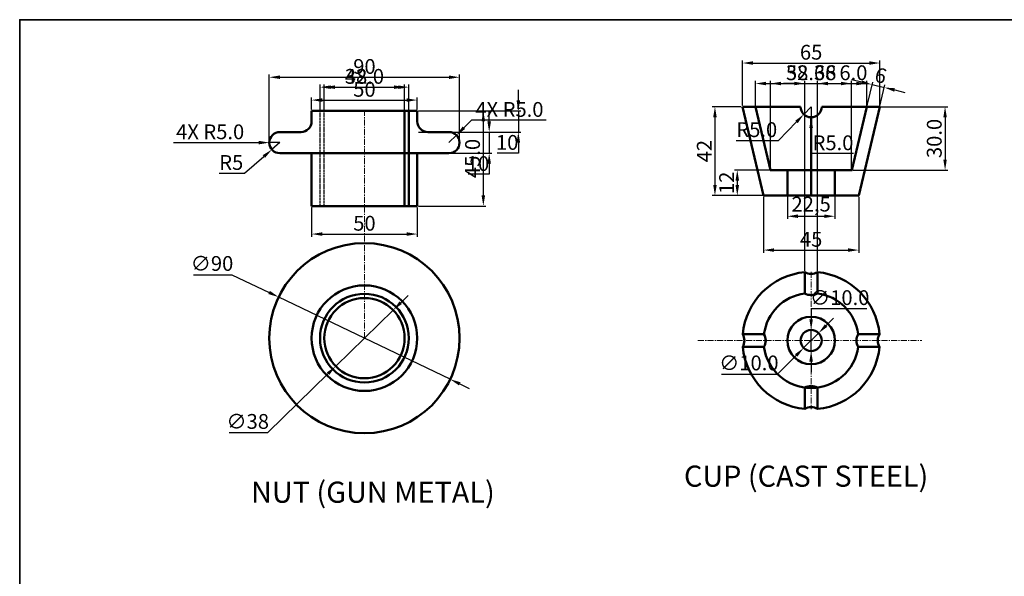
# Model space of a CAD drawing. Units: millimetres. Extents: x 4274 to 5106, y 2129 to 2785.
# Tile 2 of 4: x 4274 to 4740, y 2522 to 2785. Entities that reach past the tile are written whole.
import ezdxf

# ---------------------------------------------------------------- set-up
doc = ezdxf.new("R2010")
doc.units = ezdxf.units.MM
doc.header["$LTSCALE"] = 0.3
doc.linetypes.add('ACAD_ISO02W100', pattern=[15, 12, -3])
doc.linetypes.add('CENTER', pattern=[50.8, 31.75, -6.35, 6.35, -6.35])
for name, color, linetype, lineweight in [('M-CNTR', 1, 'CENTER', 18), ('M-DIMS', 2, 'Continuous', 25), ('M-HIDN', 8, 'ACAD_ISO02W100', 25), ('M-OUTL', 7, 'Continuous', 50), ('M-TEXT', 3, 'Continuous', 25), ('M-TTLB', 7, 'Continuous', 35)]:
    doc.layers.add(name, color=color, linetype=linetype, lineweight=lineweight)
doc.styles.get("Standard").update_dxf_attribs({"font": 'arial.ttf'})
doc.dimstyles.new('ISO-25', dxfattribs={"dimtxt": 7, "dimasz": 5, "dimexe": 1.25, "dimexo": 0.625, "dimtad": 1, "dimtoh": 1, "dimtxsty": 'Standard', "dimcen": 2.5, "dimadec": 0, "dimazin": 0, "dimtfac": 1, "dimtmove": 0, "dimatfit": 3, "dimfxl": 1, "dimarcsym": 0})

# ---------------------------------------------------------------- blocks, each defined once
blk = doc.blocks.new('*D10')
at = {"layer": 'Defpoints', "color": 0, "ltscale": 0.3, "transparency": 16777216}
for p in [(4482.08, 2757.92), (4392.08, 2726.98), (4482.08, 2726.98)]:
    blk.add_point(p, dxfattribs=at)
at = {"layer": 'M-DIMS', "color": 0, "lineweight": -2, "ltscale": 0.3, "transparency": 16777216}
for p, q in [((4392.08, 2727.6), (4392.08, 2759.17)), ((4482.08, 2727.6), (4482.08, 2759.17)), ((4397.08, 2757.92), (4477.08, 2757.92))]:
    blk.add_line(p, q, dxfattribs=at)
at = {"layer": 'M-DIMS', "color": 0, "ltscale": 0.3, "transparency": 16777216}
for points in [[(4397.08, 2758.76), (4397.08, 2757.09), (4392.08, 2757.92)], [(4477.08, 2758.76), (4477.08, 2757.09), (4482.08, 2757.92)]]:
    blk.add_solid(points, dxfattribs=at)
at = {"layer": 'M-DIMS', "color": 0, "ltscale": 0.3, "transparency": 16777216, "insert": (4437.08, 2762.12), "char_height": 7, "attachment_point": 5}
blk.add_mtext('90', dxfattribs=at)
blk = doc.blocks.new('*D11')
at = {"layer": 'Defpoints', "color": 0, "ltscale": 0.3, "transparency": 16777216}
for p in [(4462.08, 2747.11), (4412.08, 2741.98), (4462.08, 2741.98)]:
    blk.add_point(p, dxfattribs=at)
at = {"layer": 'M-DIMS', "color": 0, "lineweight": -2, "ltscale": 0.3, "transparency": 16777216}
for p, q in [((4412.08, 2742.6), (4412.08, 2748.36)), ((4417.08, 2747.11), (4457.08, 2747.11)), ((4462.08, 2742.6), (4462.08, 2748.36))]:
    blk.add_line(p, q, dxfattribs=at)
at = {"layer": 'M-DIMS', "color": 0, "ltscale": 0.3, "transparency": 16777216}
for points in [[(4417.08, 2747.95), (4417.08, 2746.28), (4412.08, 2747.11)], [(4457.08, 2747.95), (4457.08, 2746.28), (4462.08, 2747.11)]]:
    blk.add_solid(points, dxfattribs=at)
at = {"layer": 'M-DIMS', "color": 0, "ltscale": 0.3, "transparency": 16777216, "insert": (4437.08, 2751.31), "char_height": 7, "attachment_point": 5}
blk.add_mtext('50', dxfattribs=at)
blk = doc.blocks.new('*D12')
at = {"layer": 'Defpoints', "color": 0, "ltscale": 0.3, "transparency": 16777216}
for p in [(4412.08, 2696.98), (4462.08, 2696.98), (4462.08, 2683.71)]:
    blk.add_point(p, dxfattribs=at)
at = {"layer": 'M-DIMS', "color": 0, "lineweight": -2, "ltscale": 0.3, "transparency": 16777216}
for p, q in [((4412.08, 2696.35), (4412.08, 2682.46)), ((4462.08, 2696.35), (4462.08, 2682.46)), ((4417.08, 2683.71), (4457.08, 2683.71))]:
    blk.add_line(p, q, dxfattribs=at)
at = {"layer": 'M-DIMS', "color": 0, "ltscale": 0.3, "transparency": 16777216}
for points in [[(4417.08, 2684.54), (4417.08, 2682.88), (4412.08, 2683.71)], [(4457.08, 2684.54), (4457.08, 2682.88), (4462.08, 2683.71)]]:
    blk.add_solid(points, dxfattribs=at)
at = {"layer": 'M-DIMS', "color": 0, "ltscale": 0.3, "transparency": 16777216, "insert": (4437.08, 2687.91), "char_height": 7, "attachment_point": 5}
blk.add_mtext('50', dxfattribs=at)
blk = doc.blocks.new('*D13')
at = {"layer": 'Defpoints', "color": 0, "ltscale": 0.3, "transparency": 16777216}
for p in [(4397.08, 2726.98), (4393.3, 2723.7)]:
    blk.add_point(p, dxfattribs=at)
at = {"layer": 'M-DIMS', "color": 0, "lineweight": -2, "ltscale": 0.3, "transparency": 16777216}
for p, q in [((4397.08, 2726.98), (4393.3, 2723.7)), ((4380.36, 2712.5), (4389.52, 2720.43)), ((4368.39, 2712.5), (4380.36, 2712.5))]:
    blk.add_line(p, q, dxfattribs=at)
at = {"layer": 'M-DIMS', "color": 0, "ltscale": 0.3, "transparency": 16777216}
blk.add_solid([(4388.97, 2721.06), (4390.06, 2719.8), (4393.3, 2723.7)], dxfattribs=at)
at = {"layer": 'M-DIMS', "color": 0, "ltscale": 0.3, "transparency": 16777216, "insert": (4374.06, 2716.68), "char_height": 7, "attachment_point": 5}
blk.add_mtext('R5', dxfattribs=at)
blk = doc.blocks.new('*D14')
at = {"layer": 'Defpoints', "color": 0, "ltscale": 0.3, "transparency": 16777216}
for p in [(4477.08, 2731.98), (4477.08, 2721.98), (4496.11, 2721.98)]:
    blk.add_point(p, dxfattribs=at)
at = {"layer": 'M-DIMS', "color": 0, "lineweight": -2, "ltscale": 0.3, "transparency": 16777216}
for p, q in [((4496.11, 2736.98), (4496.11, 2741.98)), ((4477.7, 2731.98), (4497.36, 2731.98)), ((4496.11, 2731.98), (4496.11, 2721.98)), ((4477.7, 2721.98), (4497.36, 2721.98)), ((4496.11, 2716.98), (4496.11, 2711.98)), ((4496.11, 2711.98), (4486.14, 2711.98))]:
    blk.add_line(p, q, dxfattribs=at)
at = {"layer": 'M-DIMS', "color": 0, "ltscale": 0.3, "transparency": 16777216}
for points in [[(4495.28, 2736.98), (4496.94, 2736.98), (4496.11, 2731.98)], [(4495.28, 2716.98), (4496.94, 2716.98), (4496.11, 2721.98)]]:
    blk.add_solid(points, dxfattribs=at)
at = {"layer": 'M-DIMS', "color": 0, "ltscale": 0.3, "transparency": 16777216, "insert": (4490.81, 2716.17), "char_height": 7, "attachment_point": 5}
blk.add_mtext('10', dxfattribs=at)
blk = doc.blocks.new('*D15')
at = {"layer": 'Defpoints', "color": 0, "ltscale": 0.3, "transparency": 16777216}
for p in [(4462.08, 2741.98), (4462.08, 2731.98), (4509.9, 2731.98)]:
    blk.add_point(p, dxfattribs=at)
at = {"layer": 'M-DIMS', "color": 0, "lineweight": -2, "ltscale": 0.3, "transparency": 16777216}
for p, q in [((4509.9, 2746.98), (4509.9, 2751.98)), ((4462.7, 2741.98), (4511.15, 2741.98)), ((4509.9, 2741.98), (4509.9, 2731.98)), ((4462.7, 2731.98), (4511.15, 2731.98)), ((4509.9, 2726.98), (4509.9, 2721.98)), ((4509.9, 2721.98), (4499.94, 2721.98))]:
    blk.add_line(p, q, dxfattribs=at)
at = {"layer": 'M-DIMS', "color": 0, "ltscale": 0.3, "transparency": 16777216}
for points in [[(4509.07, 2746.98), (4510.74, 2746.98), (4509.9, 2741.98)], [(4509.07, 2726.98), (4510.74, 2726.98), (4509.9, 2731.98)]]:
    blk.add_solid(points, dxfattribs=at)
at = {"layer": 'M-DIMS', "color": 0, "ltscale": 0.3, "transparency": 16777216, "insert": (4504.61, 2726.17), "char_height": 7, "attachment_point": 5}
blk.add_mtext('10', dxfattribs=at)
blk = doc.blocks.new('*D16')
at = {"layer": 'Defpoints', "color": 0, "ltscale": 0.3, "transparency": 16777216}
for p in [(4396.5, 2653.89), (4477.66, 2614.98)]:
    blk.add_point(p, dxfattribs=at)
at = {"layer": 'M-DIMS', "color": 0, "lineweight": -2, "ltscale": 0.3, "transparency": 16777216}
for p, q in [((4356.15, 2664.48), (4374.39, 2664.48)), ((4374.39, 2664.48), (4391.99, 2656.05)), ((4477.66, 2614.98), (4396.5, 2653.89)), ((4482.17, 2612.82), (4486.67, 2610.66))]:
    blk.add_line(p, q, dxfattribs=at)
at = {"layer": 'M-DIMS', "color": 0, "ltscale": 0.3, "transparency": 16777216}
for points in [[(4392.35, 2656.8), (4391.63, 2655.3), (4396.5, 2653.89)], [(4482.53, 2613.57), (4481.81, 2612.07), (4477.66, 2614.98)]]:
    blk.add_solid(points, dxfattribs=at)
at = {"layer": 'M-DIMS', "color": 0, "ltscale": 0.3, "transparency": 16777216, "insert": (4364.96, 2668.88), "char_height": 7, "attachment_point": 5}
blk.add_mtext('∅90', dxfattribs=at)
blk = doc.blocks.new('*D17')
at = {"layer": 'Defpoints', "color": 0, "ltscale": 0.3, "transparency": 16777216}
for p in [(4450.67, 2647.71), (4423.49, 2621.16)]:
    blk.add_point(p, dxfattribs=at)
at = {"layer": 'M-DIMS', "color": 0, "lineweight": -2, "ltscale": 0.3, "transparency": 16777216}
for p, q in [((4454.25, 2651.2), (4457.82, 2654.7)), ((4450.67, 2647.71), (4423.49, 2621.16)), ((4391.3, 2589.73), (4419.91, 2617.67)), ((4373.02, 2589.73), (4391.3, 2589.73))]:
    blk.add_line(p, q, dxfattribs=at)
at = {"layer": 'M-DIMS', "color": 0, "ltscale": 0.3, "transparency": 16777216}
for points in [[(4453.67, 2651.8), (4454.83, 2650.61), (4450.67, 2647.71)], [(4419.33, 2618.26), (4420.49, 2617.07), (4423.49, 2621.16)]]:
    blk.add_solid(points, dxfattribs=at)
at = {"layer": 'M-DIMS', "color": 0, "ltscale": 0.3, "transparency": 16777216, "insert": (4381.85, 2594.12), "char_height": 7, "attachment_point": 5}
blk.add_mtext('∅38', dxfattribs=at)
blk = doc.blocks.new('*D18')
at = {"layer": 'Defpoints', "color": 0, "ltscale": 0.3, "transparency": 16777216}
for p in [(4680.93, 2764.66), (4615.93, 2743.95), (4680.93, 2743.95)]:
    blk.add_point(p, dxfattribs=at)
at = {"layer": 'M-DIMS', "color": 0, "lineweight": -2, "ltscale": 0.3, "transparency": 16777216}
for p, q in [((4615.93, 2744.58), (4615.93, 2765.91)), ((4620.93, 2764.66), (4675.93, 2764.66)), ((4680.93, 2744.58), (4680.93, 2765.91))]:
    blk.add_line(p, q, dxfattribs=at)
at = {"layer": 'M-DIMS', "color": 0, "ltscale": 0.3, "transparency": 16777216}
for points in [[(4620.93, 2765.49), (4620.93, 2763.82), (4615.93, 2764.66)], [(4675.93, 2765.49), (4675.93, 2763.82), (4680.93, 2764.66)]]:
    blk.add_solid(points, dxfattribs=at)
at = {"layer": 'M-DIMS', "color": 0, "ltscale": 0.3, "transparency": 16777216, "insert": (4648.43, 2768.86), "char_height": 7, "attachment_point": 5}
blk.add_mtext('65', dxfattribs=at)
blk = doc.blocks.new('*D19')
at = {"layer": 'Defpoints', "color": 0, "ltscale": 0.3, "transparency": 16777216}
for p in [(4683.09, 2753.06), (4671.19, 2728.95), (4677.02, 2727.56)]:
    blk.add_point(p, dxfattribs=at)
at = {"layer": 'M-DIMS', "color": 0, "lineweight": -2, "ltscale": 0.3, "transparency": 16777216}
for p, q in [((4672.39, 2755.6), (4667.53, 2756.76)), ((4671.33, 2729.56), (4677.55, 2755.66)), ((4677.17, 2728.17), (4683.38, 2754.27)), ((4677.26, 2754.45), (4683.09, 2753.06)), ((4687.96, 2751.9), (4692.82, 2750.74))]:
    blk.add_line(p, q, dxfattribs=at)
at = {"layer": 'M-DIMS', "color": 0, "ltscale": 0.3, "transparency": 16777216}
for points in [[(4672.59, 2756.41), (4672.2, 2754.79), (4677.26, 2754.45)], [(4688.15, 2752.71), (4687.76, 2751.09), (4683.09, 2753.06)]]:
    blk.add_solid(points, dxfattribs=at)
at = {"layer": 'M-DIMS', "color": 0, "ltscale": 0.3, "transparency": 16777216, "insert": (4681.15, 2757.84), "char_height": 7, "attachment_point": 5, "rotation": 346.6075}
blk.add_mtext('6', dxfattribs=at)
blk = doc.blocks.new('*D20')
at = {"layer": 'Defpoints', "color": 0, "ltscale": 0.3, "transparency": 16777216}
for p in [(4615.93, 2743.95), (4602.92, 2701.95), (4625.93, 2701.95)]:
    blk.add_point(p, dxfattribs=at)
at = {"layer": 'M-DIMS', "color": 0, "lineweight": -2, "ltscale": 0.3, "transparency": 16777216}
for p, q in [((4615.3, 2743.95), (4601.67, 2743.95)), ((4602.92, 2738.95), (4602.92, 2706.95)), ((4625.3, 2701.95), (4601.67, 2701.95))]:
    blk.add_line(p, q, dxfattribs=at)
at = {"layer": 'M-DIMS', "color": 0, "ltscale": 0.3, "transparency": 16777216}
for points in [[(4602.09, 2738.95), (4603.76, 2738.95), (4602.92, 2743.95)], [(4602.09, 2706.95), (4603.76, 2706.95), (4602.92, 2701.95)]]:
    blk.add_solid(points, dxfattribs=at)
at = {"layer": 'M-DIMS', "color": 0, "ltscale": 0.3, "transparency": 16777216, "insert": (4598.78, 2722.95), "char_height": 7, "attachment_point": 5, "rotation": 90}
blk.add_mtext('42', dxfattribs=at)
blk = doc.blocks.new('*D21')
at = {"layer": 'Defpoints', "color": 0, "ltscale": 0.3, "transparency": 16777216}
for p in [(4637.18, 2713.95), (4613.49, 2701.95), (4637.18, 2701.95)]:
    blk.add_point(p, dxfattribs=at)
at = {"layer": 'M-DIMS', "color": 0, "lineweight": -2, "ltscale": 0.3, "transparency": 16777216}
for p, q in [((4636.55, 2713.95), (4612.24, 2713.95)), ((4613.49, 2708.95), (4613.49, 2706.95)), ((4636.55, 2701.95), (4612.24, 2701.95))]:
    blk.add_line(p, q, dxfattribs=at)
at = {"layer": 'M-DIMS', "color": 0, "ltscale": 0.3, "transparency": 16777216}
for points in [[(4612.65, 2708.95), (4614.32, 2708.95), (4613.49, 2713.95)], [(4612.65, 2706.95), (4614.32, 2706.95), (4613.49, 2701.95)]]:
    blk.add_solid(points, dxfattribs=at)
at = {"layer": 'M-DIMS', "color": 0, "ltscale": 0.3, "transparency": 16777216, "insert": (4609.35, 2707.95), "char_height": 7, "attachment_point": 5, "rotation": 90}
blk.add_mtext('12', dxfattribs=at)
blk = doc.blocks.new('*D22')
at = {"layer": 'Defpoints', "color": 0, "ltscale": 0.3, "transparency": 16777216}
for p in [(4625.93, 2701.95), (4670.93, 2701.95), (4670.93, 2676.12)]:
    blk.add_point(p, dxfattribs=at)
at = {"layer": 'M-DIMS', "color": 0, "lineweight": -2, "ltscale": 0.3, "transparency": 16777216}
for p, q in [((4625.93, 2701.33), (4625.93, 2674.87)), ((4670.93, 2701.33), (4670.93, 2674.87)), ((4630.93, 2676.12), (4665.93, 2676.12))]:
    blk.add_line(p, q, dxfattribs=at)
at = {"layer": 'M-DIMS', "color": 0, "ltscale": 0.3, "transparency": 16777216}
for points in [[(4630.93, 2676.96), (4630.93, 2675.29), (4625.93, 2676.12)], [(4665.93, 2676.96), (4665.93, 2675.29), (4670.93, 2676.12)]]:
    blk.add_solid(points, dxfattribs=at)
at = {"layer": 'M-DIMS', "color": 0, "ltscale": 0.3, "transparency": 16777216, "insert": (4648.43, 2680.31), "char_height": 7, "attachment_point": 5}
blk.add_mtext('45', dxfattribs=at)
blk = doc.blocks.new('*D23')
at = {"layer": 'Defpoints', "color": 0, "ltscale": 0.3, "transparency": 16777216}
for p in [(4637.18, 2701.95), (4659.68, 2701.95), (4659.68, 2692.13)]:
    blk.add_point(p, dxfattribs=at)
at = {"layer": 'M-DIMS', "color": 0, "lineweight": -2, "ltscale": 0.3, "transparency": 16777216}
for p, q in [((4637.18, 2701.33), (4637.18, 2690.88)), ((4659.68, 2701.33), (4659.68, 2690.88)), ((4642.18, 2692.13), (4654.68, 2692.13))]:
    blk.add_line(p, q, dxfattribs=at)
at = {"layer": 'M-DIMS', "color": 0, "ltscale": 0.3, "transparency": 16777216}
for points in [[(4642.18, 2692.97), (4642.18, 2691.3), (4637.18, 2692.13)], [(4654.68, 2692.97), (4654.68, 2691.3), (4659.68, 2692.13)]]:
    blk.add_solid(points, dxfattribs=at)
at = {"layer": 'M-DIMS', "color": 0, "ltscale": 0.3, "transparency": 16777216, "insert": (4648.43, 2696.96), "char_height": 7, "attachment_point": 5}
blk.add_mtext('22,5', dxfattribs=at)
blk = doc.blocks.new('*D53')
at = {"layer": 'Defpoints', "color": 0, "ltscale": 0.3, "transparency": 16777216}
for p in [(4462.08, 2741.98), (4462.08, 2696.98), (4493.33, 2696.98)]:
    blk.add_point(p, dxfattribs=at)
at = {"layer": 'M-DIMS', "color": 0, "lineweight": -2, "ltscale": 0.3, "transparency": 16777216}
for p, q in [((4462.7, 2741.98), (4494.58, 2741.98)), ((4493.33, 2736.98), (4493.33, 2701.98)), ((4462.7, 2696.98), (4494.58, 2696.98))]:
    blk.add_line(p, q, dxfattribs=at)
at = {"layer": 'M-DIMS', "color": 0, "ltscale": 0.3, "transparency": 16777216}
for points in [[(4492.49, 2736.98), (4494.16, 2736.98), (4493.33, 2741.98)], [(4492.49, 2701.98), (4494.16, 2701.98), (4493.33, 2696.98)]]:
    blk.add_solid(points, dxfattribs=at)
at = {"layer": 'M-DIMS', "color": 0, "ltscale": 0.3, "transparency": 16777216, "insert": (4489.13, 2719.48), "char_height": 7, "attachment_point": 5, "rotation": 90}
blk.add_mtext('45.0', dxfattribs=at)
blk = doc.blocks.new('*D54')
at = {"layer": 'Defpoints', "color": 0, "ltscale": 0.3, "transparency": 16777216}
for p in [(4456.08, 2753.23), (4418.08, 2741.98), (4456.08, 2741.98)]:
    blk.add_point(p, dxfattribs=at)
at = {"layer": 'M-DIMS', "color": 0, "lineweight": -2, "ltscale": 0.3, "transparency": 16777216}
for p, q in [((4418.08, 2742.6), (4418.08, 2754.48)), ((4456.08, 2742.6), (4456.08, 2754.48)), ((4423.08, 2753.23), (4451.08, 2753.23))]:
    blk.add_line(p, q, dxfattribs=at)
at = {"layer": 'M-DIMS', "color": 0, "ltscale": 0.3, "transparency": 16777216}
for points in [[(4423.08, 2754.06), (4423.08, 2752.39), (4418.08, 2753.23)], [(4451.08, 2754.06), (4451.08, 2752.39), (4456.08, 2753.23)]]:
    blk.add_solid(points, dxfattribs=at)
at = {"layer": 'M-DIMS', "color": 0, "ltscale": 0.3, "transparency": 16777216, "insert": (4437.08, 2757.43), "char_height": 7, "attachment_point": 5}
blk.add_mtext('38.0', dxfattribs=at)
blk = doc.blocks.new('*D55')
at = {"layer": 'Defpoints', "color": 0, "ltscale": 0.3, "transparency": 16777216}
for p in [(4458.08, 2753.23), (4416.08, 2741.98), (4458.08, 2741.98)]:
    blk.add_point(p, dxfattribs=at)
at = {"layer": 'M-DIMS', "color": 0, "lineweight": -2, "ltscale": 0.3, "transparency": 16777216}
for p, q in [((4416.08, 2742.6), (4416.08, 2754.48)), ((4458.08, 2742.6), (4458.08, 2754.48)), ((4421.08, 2753.23), (4453.08, 2753.23))]:
    blk.add_line(p, q, dxfattribs=at)
at = {"layer": 'M-DIMS', "color": 0, "ltscale": 0.3, "transparency": 16777216}
for points in [[(4421.08, 2754.06), (4421.08, 2752.39), (4416.08, 2753.23)], [(4453.08, 2754.06), (4453.08, 2752.39), (4458.08, 2753.23)]]:
    blk.add_solid(points, dxfattribs=at)
at = {"layer": 'M-DIMS', "color": 0, "ltscale": 0.3, "transparency": 16777216, "insert": (4437.08, 2757.42), "char_height": 7, "attachment_point": 5}
blk.add_mtext('42.0', dxfattribs=at)
blk = doc.blocks.new('*D56')
at = {"layer": 'Defpoints', "color": 0, "ltscale": 0.3, "transparency": 16777216}
for p in [(4667.61, 2754.95), (4629.24, 2713.95), (4667.61, 2713.95)]:
    blk.add_point(p, dxfattribs=at)
at = {"layer": 'M-DIMS', "color": 0, "lineweight": -2, "ltscale": 0.3, "transparency": 16777216}
for p, q in [((4629.24, 2714.58), (4629.24, 2756.2)), ((4634.24, 2754.95), (4662.61, 2754.95)), ((4667.61, 2714.58), (4667.61, 2756.2))]:
    blk.add_line(p, q, dxfattribs=at)
at = {"layer": 'M-DIMS', "color": 0, "ltscale": 0.3, "transparency": 16777216}
for points in [[(4634.24, 2755.78), (4634.24, 2754.12), (4629.24, 2754.95)], [(4662.61, 2755.78), (4662.61, 2754.12), (4667.61, 2754.95)]]:
    blk.add_solid(points, dxfattribs=at)
at = {"layer": 'M-DIMS', "color": 0, "ltscale": 0.3, "transparency": 16777216, "insert": (4648.43, 2759.15), "char_height": 7, "attachment_point": 5}
blk.add_mtext('38.38', dxfattribs=at)
blk = doc.blocks.new('*D57')
at = {"layer": 'Defpoints', "color": 0, "ltscale": 0.3, "transparency": 16777216}
for p in [(4674.76, 2754.95), (4622.09, 2743.95), (4674.76, 2743.95)]:
    blk.add_point(p, dxfattribs=at)
at = {"layer": 'M-DIMS', "color": 0, "lineweight": -2, "ltscale": 0.3, "transparency": 16777216}
for p, q in [((4622.09, 2744.58), (4622.09, 2756.2)), ((4627.09, 2754.95), (4669.76, 2754.95)), ((4674.76, 2744.58), (4674.76, 2756.2))]:
    blk.add_line(p, q, dxfattribs=at)
at = {"layer": 'M-DIMS', "color": 0, "ltscale": 0.3, "transparency": 16777216}
for points in [[(4627.09, 2755.78), (4627.09, 2754.12), (4622.09, 2754.95)], [(4669.76, 2755.78), (4669.76, 2754.12), (4674.76, 2754.95)]]:
    blk.add_solid(points, dxfattribs=at)
at = {"layer": 'M-DIMS', "color": 0, "ltscale": 0.3, "transparency": 16777216, "insert": (4648.43, 2759.15), "char_height": 7, "attachment_point": 5}
blk.add_mtext('52.66', dxfattribs=at)
blk = doc.blocks.new('*D58')
at = {"layer": 'Defpoints', "color": 0, "ltscale": 0.3, "transparency": 16777216}
for p in [(4674.76, 2743.95), (4667.61, 2713.95), (4711.8, 2713.95)]:
    blk.add_point(p, dxfattribs=at)
at = {"layer": 'M-DIMS', "color": 0, "lineweight": -2, "ltscale": 0.3, "transparency": 16777216}
for p, q in [((4675.38, 2743.95), (4713.05, 2743.95)), ((4711.8, 2738.95), (4711.8, 2718.95)), ((4668.24, 2713.95), (4713.05, 2713.95))]:
    blk.add_line(p, q, dxfattribs=at)
at = {"layer": 'M-DIMS', "color": 0, "ltscale": 0.3, "transparency": 16777216}
for points in [[(4710.97, 2738.95), (4712.63, 2738.95), (4711.8, 2743.95)], [(4710.97, 2718.95), (4712.63, 2718.95), (4711.8, 2713.95)]]:
    blk.add_solid(points, dxfattribs=at)
at = {"layer": 'M-DIMS', "color": 0, "ltscale": 0.3, "transparency": 16777216, "insert": (4707.6, 2728.95), "char_height": 7, "attachment_point": 5, "rotation": 90}
blk.add_mtext('30.0', dxfattribs=at)
blk = doc.blocks.new('*D59')
at = {"layer": 'Defpoints', "color": 0, "ltscale": 0.3, "transparency": 16777216}
for p in [(4651.43, 2754.95), (4645.43, 2665.68), (4651.43, 2665.68)]:
    blk.add_point(p, dxfattribs=at)
at = {"layer": 'M-DIMS', "color": 0, "lineweight": -2, "ltscale": 0.3, "transparency": 16777216}
for p, q in [((4640.43, 2754.95), (4635.43, 2754.95)), ((4645.43, 2666.3), (4645.43, 2756.2)), ((4645.43, 2754.95), (4651.43, 2754.95)), ((4651.43, 2666.3), (4651.43, 2756.2)), ((4656.43, 2754.95), (4675.43, 2754.95))]:
    blk.add_line(p, q, dxfattribs=at)
at = {"layer": 'M-DIMS', "color": 0, "ltscale": 0.3, "transparency": 16777216}
for points in [[(4640.43, 2755.78), (4640.43, 2754.12), (4645.43, 2754.95)], [(4656.43, 2755.78), (4656.43, 2754.12), (4651.43, 2754.95)]]:
    blk.add_solid(points, dxfattribs=at)
at = {"layer": 'M-DIMS', "color": 0, "ltscale": 0.3, "transparency": 16777216, "insert": (4668.43, 2759.15), "char_height": 7, "attachment_point": 5}
blk.add_mtext('6.0', dxfattribs=at)
blk = doc.blocks.new('*D70')
at = {"layer": 'Defpoints', "color": 0, "ltscale": 0.3, "transparency": 16777216}
for p in [(4392.08, 2726.98), (4397.08, 2726.98)]:
    blk.add_point(p, dxfattribs=at)
at = {"layer": 'M-DIMS', "color": 0, "lineweight": -2, "ltscale": 0.3, "transparency": 16777216}
for p, q in [((4346.71, 2726.99), (4382.08, 2726.99)), ((4382.08, 2726.99), (4387.08, 2726.98)), ((4397.08, 2726.98), (4392.08, 2726.98))]:
    blk.add_line(p, q, dxfattribs=at)
at = {"layer": 'M-DIMS', "color": 0, "ltscale": 0.3, "transparency": 16777216}
blk.add_solid([(4387.08, 2727.82), (4387.08, 2726.15), (4392.08, 2726.98)], dxfattribs=at)
at = {"layer": 'M-DIMS', "color": 0, "ltscale": 0.3, "transparency": 16777216, "insert": (4364.08, 2731.19), "char_height": 7, "attachment_point": 5}
blk.add_mtext('4X R5.0', dxfattribs=at)
blk = doc.blocks.new('*D71')
at = {"layer": 'Defpoints', "color": 0, "ltscale": 0.3, "transparency": 16777216}
for p in [(4648.43, 2743.95), (4648.43, 2738.95)]:
    blk.add_point(p, dxfattribs=at)
at = {"layer": 'M-DIMS', "color": 0, "lineweight": -2, "ltscale": 0.3, "transparency": 16777216}
for p, q in [((4648.43, 2743.95), (4648.43, 2738.95)), ((4648.45, 2721.8), (4648.43, 2733.95)), ((4668.49, 2721.8), (4648.45, 2721.8))]:
    blk.add_line(p, q, dxfattribs=at)
at = {"layer": 'M-DIMS', "color": 0, "ltscale": 0.3, "transparency": 16777216}
blk.add_solid([(4649.27, 2733.95), (4647.6, 2733.95), (4648.43, 2738.95)], dxfattribs=at)
at = {"layer": 'M-DIMS', "color": 0, "ltscale": 0.3, "transparency": 16777216, "insert": (4658.78, 2726), "char_height": 7, "attachment_point": 5}
blk.add_mtext('R5.0', dxfattribs=at)
blk = doc.blocks.new('*D72')
at = {"layer": 'Defpoints', "color": 0, "ltscale": 0.3, "transparency": 16777216}
for p in [(4648.43, 2638.32), (4648.42, 2628.32)]:
    blk.add_point(p, dxfattribs=at)
at = {"layer": 'M-DIMS', "color": 0, "lineweight": -2, "ltscale": 0.3, "transparency": 16777216}
for p, q in [((4648.44, 2648.32), (4648.43, 2643.32)), ((4674.84, 2648.32), (4648.44, 2648.32)), ((4648.42, 2628.32), (4648.43, 2638.32)), ((4648.42, 2623.32), (4648.41, 2618.32))]:
    blk.add_line(p, q, dxfattribs=at)
at = {"layer": 'M-DIMS', "color": 0, "ltscale": 0.3, "transparency": 16777216}
for points in [[(4647.6, 2643.32), (4649.27, 2643.32), (4648.43, 2638.32)], [(4647.58, 2623.32), (4649.25, 2623.32), (4648.42, 2628.32)]]:
    blk.add_solid(points, dxfattribs=at)
at = {"layer": 'M-DIMS', "color": 0, "ltscale": 0.3, "transparency": 16777216, "insert": (4661.95, 2652.71), "char_height": 7, "attachment_point": 5}
blk.add_mtext('∅10.0', dxfattribs=at)
blk = doc.blocks.new('*D87')
at = {"layer": 'Defpoints', "color": 0, "ltscale": 0.3, "transparency": 16777216}
for p in [(4480.61, 2730.51), (4477.08, 2726.98)]:
    blk.add_point(p, dxfattribs=at)
at = {"layer": 'M-DIMS', "color": 0, "lineweight": -2, "ltscale": 0.3, "transparency": 16777216}
for p, q in [((4487.68, 2737.59), (4484.15, 2734.05)), ((4523.05, 2737.59), (4487.68, 2737.59)), ((4477.08, 2726.98), (4480.61, 2730.51))]:
    blk.add_line(p, q, dxfattribs=at)
at = {"layer": 'M-DIMS', "color": 0, "ltscale": 0.3, "transparency": 16777216}
blk.add_solid([(4483.56, 2734.64), (4484.74, 2733.46), (4480.61, 2730.51)], dxfattribs=at)
at = {"layer": 'M-DIMS', "color": 0, "ltscale": 0.3, "transparency": 16777216, "insert": (4505.68, 2741.78), "char_height": 7, "attachment_point": 5}
blk.add_mtext('4X R5.0', dxfattribs=at)
blk = doc.blocks.new('*D88')
at = {"layer": 'Defpoints', "color": 0, "ltscale": 0.3, "transparency": 16777216}
for p in [(4644.95, 2740.35), (4648.43, 2743.95)]:
    blk.add_point(p, dxfattribs=at)
at = {"layer": 'M-DIMS', "color": 0, "lineweight": -2, "ltscale": 0.3, "transparency": 16777216}
for p, q in [((4648.43, 2743.95), (4644.95, 2740.35)), ((4633.05, 2728.01), (4641.48, 2736.75)), ((4613, 2728.01), (4633.05, 2728.01))]:
    blk.add_line(p, q, dxfattribs=at)
at = {"layer": 'M-DIMS', "color": 0, "ltscale": 0.3, "transparency": 16777216}
blk.add_solid([(4640.88, 2737.33), (4642.08, 2736.18), (4644.95, 2740.35)], dxfattribs=at)
at = {"layer": 'M-DIMS', "color": 0, "ltscale": 0.3, "transparency": 16777216, "insert": (4622.71, 2732.21), "char_height": 7, "attachment_point": 5}
blk.add_mtext('R5.0', dxfattribs=at)
blk = doc.blocks.new('*D89')
at = {"layer": 'Defpoints', "color": 0, "ltscale": 0.3, "transparency": 16777216}
for p in [(4651.97, 2636.85), (4644.89, 2629.79)]:
    blk.add_point(p, dxfattribs=at)
at = {"layer": 'M-DIMS', "color": 0, "lineweight": -2, "ltscale": 0.3, "transparency": 16777216}
for p, q in [((4655.51, 2640.38), (4659.04, 2643.91)), ((4651.97, 2636.85), (4644.89, 2629.79)), ((4632.47, 2617.4), (4641.35, 2626.25)), ((4606.07, 2617.4), (4632.47, 2617.4))]:
    blk.add_line(p, q, dxfattribs=at)
at = {"layer": 'M-DIMS', "color": 0, "ltscale": 0.3, "transparency": 16777216}
for points in [[(4654.92, 2640.97), (4656.09, 2639.79), (4651.97, 2636.85)], [(4640.76, 2626.84), (4641.93, 2625.66), (4644.89, 2629.79)]]:
    blk.add_solid(points, dxfattribs=at)
at = {"layer": 'M-DIMS', "color": 0, "ltscale": 0.3, "transparency": 16777216, "insert": (4618.96, 2621.79), "char_height": 7, "attachment_point": 5}
blk.add_mtext('∅10.0', dxfattribs=at)

msp = doc.modelspace()

# ---------------------------------------------------------------- linework, layer by layer
at = {"layer": 'M-CNTR', "ltscale": 0.3}
for p, q in [((4437.0779, 2634.4352), (4437.0779, 2741.9752)), ((4648.4255, 2665.817), (4648.4255, 2600.817)), ((4594.8615, 2633.317), (4700.8, 2633.317))]:
    msp.add_line(p, q, dxfattribs=at)
at = {"layer": 'M-HIDN', "ltscale": 0.3}
for p, q in [((4416.0779, 2696.9752), (4416.0779, 2741.9752)), ((4418.0779, 2696.9752), (4418.0779, 2741.9752))]:
    msp.add_line(p, q, dxfattribs=at)
at = {"layer": 'M-OUTL', "ltscale": 0.3}
for p, q in [((4437.0779, 2741.9752), (4412.0779, 2741.9752)), ((4437.0779, 2741.9752), (4412.0779, 2741.9752)), ((4412.0779, 2741.9752), (4412.0779, 2736.9752)), ((4437.0779, 2741.9752), (4462.0779, 2741.9752)), ((4456.0779, 2696.9752), (4456.0779, 2741.9752)), ((4458.0779, 2696.9752), (4458.0779, 2741.9752)), ((4462.0779, 2736.9752), (4462.0779, 2741.9752)), ((4615.9255, 2743.9507), (4625.9255, 2701.9507)), ((4643.4255, 2743.9507), (4615.9255, 2743.9507)), ((4622.0932, 2743.9507), (4629.2361, 2713.9507)), ((4643.4255, 2743.9507), (4625.9255, 2743.9507)), ((4653.4255, 2743.9507), (4680.9255, 2743.9507)), ((4680.9255, 2743.9507), (4653.4255, 2743.9507)), ((4667.6149, 2713.9507), (4674.7578, 2743.9507)), ((4670.9255, 2701.9507), (4680.9255, 2743.9507)), ((4648.4255, 2738.9507), (4648.4255, 2701.9507)), ((4397.0779, 2731.9752), (4407.0779, 2731.9752)), ((4467.0779, 2731.9752), (4477.0779, 2731.9752)), ((4397.0779, 2721.9752), (4477.0779, 2721.9752)), ((4412.0779, 2721.9752), (4412.0779, 2696.9752)), ((4462.0779, 2696.9752), (4462.0779, 2721.9752)), ((4629.0684, 2713.9507), (4667.7826, 2713.9507)), ((4659.6755, 2713.9507), (4637.1755, 2713.9507)), ((4637.1755, 2713.9507), (4637.1755, 2701.9507)), ((4659.6755, 2713.9507), (4659.6755, 2701.9507)), ((4648.4255, 2701.9507), (4625.9255, 2701.9507)), ((4625.9255, 2701.9507), (4670.9255, 2701.9507)), ((4659.6755, 2701.9507), (4637.1755, 2701.9507)), ((4648.4255, 2701.9507), (4670.9255, 2701.9507)), ((4648.4255, 2701.9507), (4659.6755, 2701.9507)), ((4412.0779, 2696.9752), (4462.0779, 2696.9752)), ((4645.4255, 2665.6783), (4645.4255, 2655.6162)), ((4651.4255, 2665.6783), (4651.4255, 2655.6162)), ((4616.0643, 2636.317), (4626.1264, 2636.317)), ((4680.7867, 2636.317), (4670.7246, 2636.317)), ((4616.0643, 2630.317), (4626.1264, 2630.317)), ((4680.7867, 2630.317), (4670.7246, 2630.317)), ((4645.4255, 2600.9558), (4645.4255, 2611.0179)), ((4645.4255, 2611.0179), (4645.4255, 2600.9558)), ((4651.4255, 2600.9558), (4651.4255, 2611.0179)), ((4651.4255, 2611.0179), (4651.4255, 2600.9558))]:
    msp.add_line(p, q, dxfattribs=at)
for centre, radius in [((4437.0779, 2634.4352), 45), ((4437.0779, 2634.4352), 25), ((4437.0779, 2634.4352), 21), ((4437.0779, 2634.4352), 19), ((4648.4255, 2633.317), 11.25), ((4648.4255, 2633.317), 5)]:
    msp.add_circle(centre, radius, dxfattribs=at)
for centre, radius, start, end in [((4648.4255, 2743.9507), 5, 180, 0), ((4407.0779, 2736.9752), 5, 270, 0), ((4467.0779, 2736.9752), 5, 180, 270), ((4397.0779, 2726.9752), 5, 90, 270), ((4477.0779, 2726.9752), 5, 270, 90), ((4648.4255, 2633.317), 32.5, 95.296381, 174.703619), ((4648.4255, 2670.8744), 6, 240, 300), ((4648.4255, 2633.317), 32.5, 5.296381, 84.703619), ((4648.4255, 2633.317), 22.5, 97.662256, 172.337744), ((4648.4255, 2660.8123), 6, 240, 300), ((4648.4255, 2633.317), 22.5, 7.662256, 82.337744), ((4610.8681, 2633.317), 6, 330, 30), ((4620.9302, 2633.317), 6, 330, 30), ((4675.9208, 2633.317), 6, 150, 210), ((4685.9829, 2633.317), 6, 150, 210), ((4648.4255, 2633.317), 32.5, 185.296381, 264.703619), ((4648.4255, 2633.317), 22.5, 187.662256, 352.337744), ((4648.4255, 2633.317), 32.5, 275.296381, 354.703619), ((4648.4255, 2605.8218), 6, 60, 120), ((4648.4255, 2595.7597), 6, 60, 120)]:
    msp.add_arc(centre, radius, start, end, dxfattribs=at)
at = {"layer": 'M-TTLB', "ltscale": 0.3}
msp.add_lwpolyline([(5077.4601, 2139.9092), (4273.9655, 2139.9092), (4273.9655, 2785.1666), (5077.4601, 2785.1666)], close=True, dxfattribs=at)

# ---------------------------------------------------------------- texts
at = {"layer": 'M-TEXT', "ltscale": 0.3, "char_height": 10, "attachment_point": 1}
for s, width, insert in [('CUP (CAST STEEL)', 131.81659, (4588.2651, 2574.124)), ('NUT (GUN METAL)', 126.863962, (4383.4379, 2566.5278))]:
    msp.add_mtext_dynamic_manual_height_columns(s, width=width, gutter_width=12.5, heights=[0], dxfattribs=dict(at, insert=insert))

# ---------------------------------------------------------------- dimensions: what is measured, and where the dimension line sits
at = {"layer": 'M-DIMS', "ltscale": 0.3}
dim = msp.add_linear_dim(base=(4680.9255, 2764.6565), p1=(4615.9255, 2743.9507), p2=(4680.9255, 2743.9507), dimstyle='ISO-25', override={"dimclrd": 0, "dimclre": 0, "dimclrt": 0}, dxfattribs=at)
dim.commit()
dim.dimension.update_dxf_attribs({"geometry": '*D18', "text_midpoint": (4648.4255, 2764.6565), "dimtype": 160})
for base, p1, p2, override, picture, middle in [((4482.0779, 2757.9235), (4392.0779, 2726.9752), (4482.0779, 2726.9752), {"dimclrd": 0, "dimclre": 0, "dimclrt": 0}, '*D10', (4437.0779, 2762.1225)), ((4674.7578, 2754.9507), (4622.0932, 2743.9507), (4674.7578, 2743.9507), {"dimdec": 2, "dimlfac": 1, "dimrnd": 0, "dimzin": 0, "dimdsep": 46, "dimlunit": 2}, '*D57', (4648.4255, 2759.1498)), ((4667.6149, 2754.9507), (4629.2361, 2713.9507), (4667.6149, 2713.9507), {"dimdec": 2, "dimlfac": 1, "dimrnd": 0, "dimzin": 0, "dimdsep": 46, "dimlunit": 2}, '*D56', (4648.4255, 2759.1521)), ((4651.4255, 2754.9507), (4645.4255, 2665.6783), (4651.4255, 2665.6783), {"dimdec": 1, "dimlfac": 1, "dimrnd": 0, "dimzin": 0, "dimdsep": 46, "dimlunit": 2}, '*D59', (4668.4298, 2759.1498)), ((4458.0779, 2753.2252), (4416.0779, 2741.9752), (4458.0779, 2741.9752), {"dimdec": 1, "dimlfac": 1, "dimrnd": 0, "dimzin": 0, "dimdsep": 46, "dimlunit": 2}, '*D55', (4437.0779, 2757.4242)), ((4456.0779, 2753.2252), (4418.0779, 2741.9752), (4456.0779, 2741.9752), {"dimdec": 1, "dimlfac": 1, "dimrnd": 0, "dimzin": 0, "dimdsep": 46, "dimlunit": 2}, '*D54', (4437.0779, 2757.4266)), ((4462.0779, 2747.1133), (4412.0779, 2741.9752), (4462.0779, 2741.9752), {"dimclrd": 0, "dimclre": 0, "dimclrt": 0}, '*D11', (4437.0779, 2751.3123)), ((4670.9255, 2676.1229), (4625.9255, 2701.9507), (4670.9255, 2701.9507), {"dimclrd": 0, "dimclre": 0, "dimclrt": 0}, '*D22', (4648.4255, 2680.3076)), ((4659.6755, 2692.1324), (4637.1755, 2701.9507), (4659.6755, 2701.9507), {"dimclrd": 0, "dimclre": 0, "dimclrt": 0}, '*D23', (4648.4255, 2696.964)), ((4462.0779, 2683.7109), (4412.0779, 2696.9752), (4462.0779, 2696.9752), {"dimclrd": 0, "dimclre": 0, "dimclrt": 0}, '*D12', (4437.0779, 2687.9099))]:
    dim = msp.add_linear_dim(base=base, p1=p1, p2=p2, dimstyle='ISO-25', override=override, dxfattribs=at)
    dim.commit()
    dim.dimension.update_dxf_attribs({"geometry": picture, "text_midpoint": middle})
for p1, p2, distance, picture, middle in [((4671.1863, 2728.9507), (4677.0232, 2727.561), 26.2077, '*D19', (4681.1476, 2757.8358)), ((4462.0779, 2741.9752), (4462.0779, 2731.9752), 47.827, '*D15', (4504.6077, 2726.1742)), ((4477.0779, 2731.9752), (4477.0779, 2721.9752), 19.0335, '*D14', (4490.8142, 2716.1742))]:
    dim = msp.add_aligned_dim(p1=p1, p2=p2, distance=distance, dimstyle='ISO-25', override={"dimclrd": 0, "dimclre": 0, "dimclrt": 0}, dxfattribs=at)
    dim.commit()
    dim.dimension.update_dxf_attribs({"geometry": picture, "text_midpoint": middle})
for center, mpoint, picture, middle in [((4477.0779, 2726.9752), (4480.6121, 2730.5121), '*D87', (4505.6765, 2741.7849)), ((4397.0779, 2726.9752), (4392.0779, 2726.98), '*D70', (4364.0819, 2731.1887))]:
    dim = msp.add_radius_dim(center=center, mpoint=mpoint, text='4X <>', dimstyle='ISO-25', override={"dimdec": 1, "dimlfac": 1, "dimrnd": 0, "dimzin": 0, "dimdsep": 46, "dimlunit": 2}, dxfattribs=at)
    dim.commit()
    dim.dimension.update_dxf_attribs({"geometry": picture, "text_midpoint": middle})
for base, p1, p2, override, picture, middle in [((4493.3279, 2696.9752), (4462.0779, 2741.9752), (4462.0779, 2696.9752), {"dimdec": 1, "dimlfac": 1, "dimrnd": 0, "dimzin": 0, "dimdsep": 46, "dimlunit": 2}, '*D53', (4489.1289, 2719.4752)), ((4602.9238, 2701.9507), (4615.9255, 2743.9507), (4625.9255, 2701.9507), {"dimclrd": 0, "dimclre": 0, "dimclrt": 0}, '*D20', (4598.7845, 2722.9507)), ((4711.8, 2713.9507), (4674.7578, 2743.9507), (4667.6149, 2713.9507), {"dimdec": 1, "dimlfac": 1, "dimrnd": 0, "dimzin": 0, "dimdsep": 46, "dimlunit": 2}, '*D58', (4707.5986, 2728.9507)), ((4613.4872, 2701.9507), (4637.1755, 2713.9507), (4637.1755, 2701.9507), {"dimclrd": 0, "dimclre": 0, "dimclrt": 0}, '*D21', (4609.3478, 2707.9507))]:
    dim = msp.add_linear_dim(base=base, p1=p1, p2=p2, angle=90, dimstyle='ISO-25', override=override, dxfattribs=at)
    dim.commit()
    dim.dimension.update_dxf_attribs({"geometry": picture, "text_midpoint": middle})
for center, mpoint, override, picture, middle in [((4648.4255, 2743.9507), (4644.954, 2740.3523), {"dimdec": 1, "dimlfac": 1, "dimrnd": 0, "dimzin": 0, "dimdsep": 46, "dimlunit": 2}, '*D88', (4622.7134, 2732.2101)), ((4648.4255, 2743.9507), (4648.43, 2738.9507), {"dimdec": 1, "dimlfac": 1, "dimrnd": 0, "dimzin": 0, "dimdsep": 46, "dimlunit": 2}, '*D71', (4658.7802, 2726.0017)), ((4397.0779, 2726.9752), (4393.2981, 2723.7022), {"dimclrd": 0, "dimclre": 0, "dimclrt": 0}, '*D13', (4374.0611, 2716.6805))]:
    dim = msp.add_radius_dim(center=center, mpoint=mpoint, dimstyle='ISO-25', override=override, dxfattribs=at)
    dim.commit()
    dim.dimension.update_dxf_attribs({"geometry": picture, "text_midpoint": middle})
for p1, p2, override, picture, middle in [((4477.657, 2614.9842), (4396.4989, 2653.8862), {"dimclrd": 0, "dimclre": 0, "dimclrt": 0}, '*D16', (4364.9568, 2664.483)), ((4648.421, 2628.317), (4648.43, 2638.317), {"dimdec": 1, "dimlfac": 1, "dimrnd": 0, "dimzin": 0, "dimdsep": 46, "dimlunit": 2}, '*D72', (4661.9515, 2648.317)), ((4450.6708, 2647.7105), (4423.4851, 2621.1599), {"dimclrd": 0, "dimclre": 0, "dimclrt": 0}, '*D17', (4381.8469, 2589.7275)), ((4651.9653, 2636.8483), (4644.8857, 2629.7858), {"dimdec": 1, "dimlfac": 1, "dimrnd": 0, "dimzin": 0, "dimdsep": 46, "dimlunit": 2}, '*D89', (4618.9561, 2617.3983))]:
    dim = msp.add_diameter_dim_2p(p1=p1, p2=p2, dimstyle='ISO-25', override=override, dxfattribs=at)
    dim.commit()
    dim.dimension.update_dxf_attribs({"geometry": picture, "text_midpoint": middle, "dimtype": 163})

doc.saveas('drawing.dxf')
